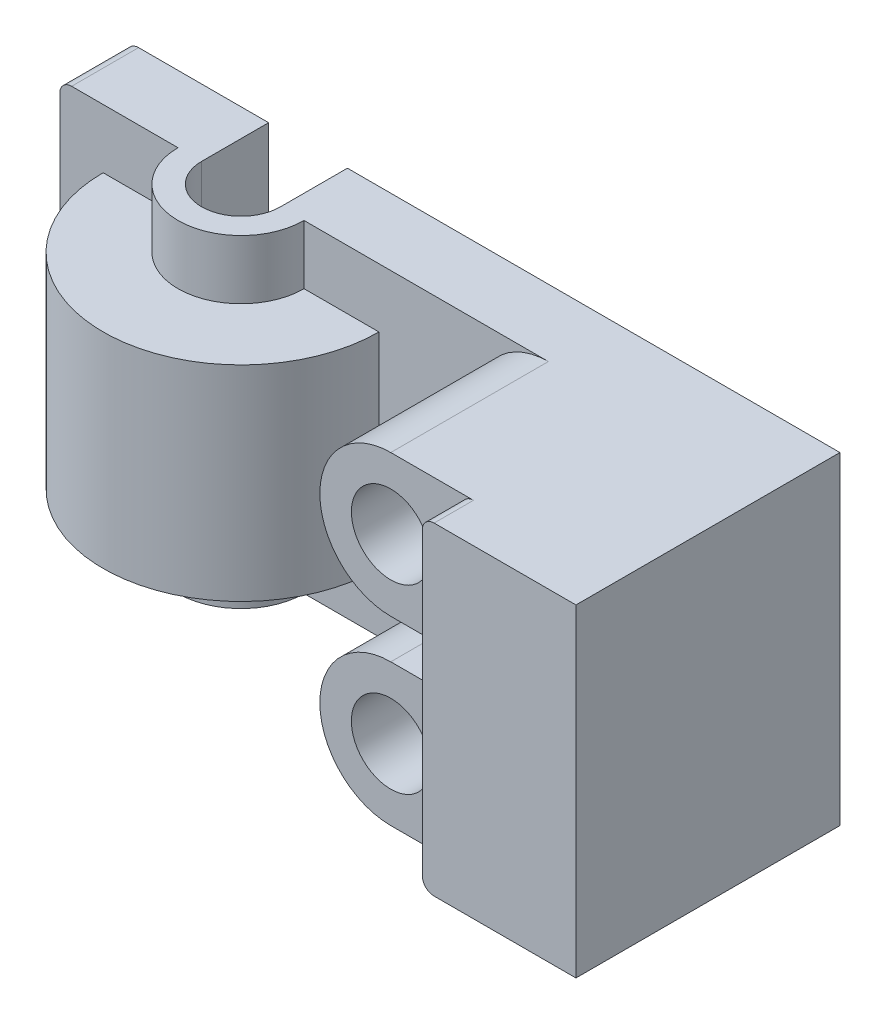
ISO-10303-21;
HEADER;
FILE_DESCRIPTION(('STEP AP214'),'2;1');
FILE_NAME('part.step','',(''),(''),'','','');
FILE_SCHEMA(('AUTOMOTIVE_DESIGN { 1 0 10303 214 1 1 1 1 }'));
ENDSEC;
DATA;
#1=APPLICATION_CONTEXT('core data for automotive mechanical design processes');
#2=APPLICATION_PROTOCOL_DEFINITION('international standard','automotive_design',2000,#1);
#3=PRODUCT_CONTEXT('',#1,'mechanical');
#4=PRODUCT('Part','Part','',(#3));
#5=PRODUCT_RELATED_PRODUCT_CATEGORY('part','',(#4));
#6=PRODUCT_DEFINITION_FORMATION('','',#4);
#7=PRODUCT_DEFINITION_CONTEXT('part definition',#1,'design');
#8=PRODUCT_DEFINITION('design','',#6,#7);
#9=PRODUCT_DEFINITION_SHAPE('','',#8);
#10=(LENGTH_UNIT() NAMED_UNIT(*) SI_UNIT(.MILLI.,.METRE.));
#11=(NAMED_UNIT(*) PLANE_ANGLE_UNIT() SI_UNIT($,.RADIAN.));
#12=(NAMED_UNIT(*) SI_UNIT($,.STERADIAN.) SOLID_ANGLE_UNIT());
#13=UNCERTAINTY_MEASURE_WITH_UNIT(LENGTH_MEASURE(1.E-05),#10,'distance_accuracy_value','');
#14=(GEOMETRIC_REPRESENTATION_CONTEXT(3) GLOBAL_UNCERTAINTY_ASSIGNED_CONTEXT((#13)) GLOBAL_UNIT_ASSIGNED_CONTEXT((#10,
#11,#12)) REPRESENTATION_CONTEXT('',''));
#15=CARTESIAN_POINT('',(0.,0.,0.));
#16=DIRECTION('',(0.,0.,1.));
#17=DIRECTION('',(1.,0.,0.));
#18=AXIS2_PLACEMENT_3D('',#15,#16,#17);
#19=CARTESIAN_POINT('',(0.,0.,17.));
#20=DIRECTION('',(0.,0.,1.));
#21=DIRECTION('',(1.,0.,0.));
#22=AXIS2_PLACEMENT_3D('',#19,#20,#21);
#23=PLANE('',#22);
#24=DIRECTION('',(1.,0.,0.));
#25=VECTOR('',#24,1.);
#26=CARTESIAN_POINT('',(118.,46.,17.));
#27=LINE('',#26,#25);
#28=CARTESIAN_POINT('',(118.,46.,17.));
#29=VERTEX_POINT('',#28);
#30=CARTESIAN_POINT('',(136.,46.,17.));
#31=VERTEX_POINT('',#30);
#32=EDGE_CURVE('E236',#29,#31,#27,.T.);
#33=ORIENTED_EDGE('',*,*,#32,.F.);
#34=CARTESIAN_POINT('',(118.,64.,17.));
#35=DIRECTION('',(0.,0.,1.));
#36=DIRECTION('',(1.,0.,0.));
#37=AXIS2_PLACEMENT_3D('',#34,#35,#36);
#38=CIRCLE('',#37,18.);
#39=CARTESIAN_POINT('',(118.,82.,17.));
#40=VERTEX_POINT('',#39);
#41=EDGE_CURVE('E566',#40,#29,#38,.T.);
#42=ORIENTED_EDGE('',*,*,#41,.F.);
#43=DIRECTION('',(-1.,0.,0.));
#44=VECTOR('',#43,1.);
#45=CARTESIAN_POINT('',(175.,82.,17.));
#46=LINE('',#45,#44);
#47=CARTESIAN_POINT('',(56.,82.,17.));
#48=VERTEX_POINT('',#47);
#49=EDGE_CURVE('E253',#40,#48,#46,.T.);
#50=ORIENTED_EDGE('',*,*,#49,.T.);
#51=DIRECTION('',(0.,-1.,0.));
#52=VECTOR('',#51,1.);
#53=CARTESIAN_POINT('',(56.,82.,17.));
#54=LINE('',#53,#52);
#55=CARTESIAN_POINT('',(56.,67.,17.));
#56=VERTEX_POINT('',#55);
#57=EDGE_CURVE('E391',#48,#56,#54,.T.);
#58=ORIENTED_EDGE('',*,*,#57,.T.);
#59=DIRECTION('',(-1.,0.,0.));
#60=VECTOR('',#59,1.);
#61=CARTESIAN_POINT('',(50.,67.,17.));
#62=LINE('',#61,#60);
#63=CARTESIAN_POINT('',(75.,67.,17.));
#64=VERTEX_POINT('',#63);
#65=EDGE_CURVE('E401',#64,#56,#62,.T.);
#66=ORIENTED_EDGE('',*,*,#65,.F.);
#67=DIRECTION('',(0.,-1.,0.));
#68=VECTOR('',#67,1.);
#69=CARTESIAN_POINT('',(75.,82.,17.));
#70=LINE('',#69,#68);
#71=CARTESIAN_POINT('',(75.,15.,17.));
#72=VERTEX_POINT('',#71);
#73=EDGE_CURVE('E285',#64,#72,#70,.T.);
#74=ORIENTED_EDGE('',*,*,#73,.T.);
#75=DIRECTION('',(1.,0.,0.));
#76=VECTOR('',#75,1.);
#77=CARTESIAN_POINT('',(50.,15.,17.));
#78=LINE('',#77,#76);
#79=CARTESIAN_POINT('',(56.,15.,17.));
#80=VERTEX_POINT('',#79);
#81=EDGE_CURVE('E415',#80,#72,#78,.T.);
#82=ORIENTED_EDGE('',*,*,#81,.F.);
#83=DIRECTION('',(0.,1.,0.));
#84=VECTOR('',#83,1.);
#85=CARTESIAN_POINT('',(56.,0.,17.));
#86=LINE('',#85,#84);
#87=CARTESIAN_POINT('',(56.,0.,17.));
#88=VERTEX_POINT('',#87);
#89=EDGE_CURVE('E383',#88,#80,#86,.T.);
#90=ORIENTED_EDGE('',*,*,#89,.F.);
#91=DIRECTION('',(1.,0.,0.));
#92=VECTOR('',#91,1.);
#93=CARTESIAN_POINT('',(0.,0.,17.));
#94=LINE('',#93,#92);
#95=CARTESIAN_POINT('',(118.,0.,17.));
#96=VERTEX_POINT('',#95);
#97=EDGE_CURVE('E251',#88,#96,#94,.T.);
#98=ORIENTED_EDGE('',*,*,#97,.T.);
#99=CARTESIAN_POINT('',(118.,18.,17.));
#100=DIRECTION('',(0.,0.,1.));
#101=DIRECTION('',(1.,0.,0.));
#102=AXIS2_PLACEMENT_3D('',#99,#100,#101);
#103=CIRCLE('',#102,18.);
#104=CARTESIAN_POINT('',(118.,36.,17.));
#105=VERTEX_POINT('',#104);
#106=EDGE_CURVE('E360',#105,#96,#103,.T.);
#107=ORIENTED_EDGE('',*,*,#106,.F.);
#108=DIRECTION('',(-1.,0.,0.));
#109=VECTOR('',#108,1.);
#110=CARTESIAN_POINT('',(118.,36.,17.));
#111=LINE('',#110,#109);
#112=CARTESIAN_POINT('',(136.,36.,17.));
#113=VERTEX_POINT('',#112);
#114=EDGE_CURVE('E366',#113,#105,#111,.T.);
#115=ORIENTED_EDGE('',*,*,#114,.F.);
#116=DIRECTION('',(0.,-1.,0.));
#117=VECTOR('',#116,1.);
#118=CARTESIAN_POINT('',(136.,79.,17.));
#119=LINE('',#118,#117);
#120=EDGE_CURVE('E322',#31,#113,#119,.T.);
#121=ORIENTED_EDGE('',*,*,#120,.F.);
#122=EDGE_LOOP('',(#33,#42,#50,#58,#66,#74,#82,#90,#98,#107,#115,#121));
#123=FACE_BOUND('',#122,.T.);
#124=ADVANCED_FACE('F50',(#123),#23,.T.);
#125=CARTESIAN_POINT('',(136.,79.,67.));
#126=DIRECTION('',(1.,0.,0.));
#127=DIRECTION('',(0.,0.,-1.));
#128=AXIS2_PLACEMENT_3D('',#125,#126,#127);
#129=PLANE('',#128);
#130=DIRECTION('',(0.,0.,-1.));
#131=VECTOR('',#130,1.);
#132=CARTESIAN_POINT('',(136.,46.,57.));
#133=LINE('',#132,#131);
#134=CARTESIAN_POINT('',(136.,46.,57.));
#135=VERTEX_POINT('',#134);
#136=EDGE_CURVE('E556',#135,#31,#133,.T.);
#137=ORIENTED_EDGE('',*,*,#136,.T.);
#138=ORIENTED_EDGE('',*,*,#120,.T.);
#139=DIRECTION('',(0.,0.,-1.));
#140=VECTOR('',#139,1.);
#141=CARTESIAN_POINT('',(136.,36.,57.));
#142=LINE('',#141,#140);
#143=CARTESIAN_POINT('',(136.,36.,57.));
#144=VERTEX_POINT('',#143);
#145=EDGE_CURVE('E351',#144,#113,#142,.T.);
#146=ORIENTED_EDGE('',*,*,#145,.F.);
#147=DIRECTION('',(0.,1.,0.));
#148=VECTOR('',#147,1.);
#149=CARTESIAN_POINT('',(136.,36.,57.));
#150=LINE('',#149,#148);
#151=CARTESIAN_POINT('',(136.,3.,57.));
#152=VERTEX_POINT('',#151);
#153=EDGE_CURVE('E353',#152,#144,#150,.T.);
#154=ORIENTED_EDGE('',*,*,#153,.F.);
#155=DIRECTION('',(0.,0.,-1.));
#156=VECTOR('',#155,1.);
#157=CARTESIAN_POINT('',(136.,3.,67.));
#158=LINE('',#157,#156);
#159=CARTESIAN_POINT('',(136.,3.,67.));
#160=VERTEX_POINT('',#159);
#161=EDGE_CURVE('E246',#160,#152,#158,.T.);
#162=ORIENTED_EDGE('',*,*,#161,.F.);
#163=DIRECTION('',(0.,-1.,0.));
#164=VECTOR('',#163,1.);
#165=CARTESIAN_POINT('',(136.,79.,67.));
#166=LINE('',#165,#164);
#167=CARTESIAN_POINT('',(136.,79.,67.));
#168=VERTEX_POINT('',#167);
#169=EDGE_CURVE('E328',#168,#160,#166,.T.);
#170=ORIENTED_EDGE('',*,*,#169,.F.);
#171=DIRECTION('',(0.,0.,-1.));
#172=VECTOR('',#171,1.);
#173=CARTESIAN_POINT('',(136.,79.,67.));
#174=LINE('',#173,#172);
#175=CARTESIAN_POINT('',(136.,79.,57.));
#176=VERTEX_POINT('',#175);
#177=EDGE_CURVE('E245',#168,#176,#174,.T.);
#178=ORIENTED_EDGE('',*,*,#177,.T.);
#179=DIRECTION('',(0.,1.,0.));
#180=VECTOR('',#179,1.);
#181=CARTESIAN_POINT('',(136.,46.,57.));
#182=LINE('',#181,#180);
#183=EDGE_CURVE('E65',#135,#176,#182,.T.);
#184=ORIENTED_EDGE('',*,*,#183,.F.);
#185=EDGE_LOOP('',(#137,#138,#146,#154,#162,#170,#178,#184));
#186=FACE_BOUND('',#185,.T.);
#187=ADVANCED_FACE('F349',(#186),#129,.F.);
#188=CARTESIAN_POINT('',(-3.,0.,17.));
#189=VERTEX_POINT('',#188);
#190=CARTESIAN_POINT('',(24.,0.,17.));
#191=VERTEX_POINT('',#190);
#192=EDGE_CURVE('E249',#189,#191,#94,.T.);
#193=ORIENTED_EDGE('',*,*,#192,.T.);
#194=DIRECTION('',(0.,1.,0.));
#195=VECTOR('',#194,1.);
#196=CARTESIAN_POINT('',(24.,0.,17.));
#197=LINE('',#196,#195);
#198=CARTESIAN_POINT('',(24.,15.,17.));
#199=VERTEX_POINT('',#198);
#200=EDGE_CURVE('E382',#191,#199,#197,.T.);
#201=ORIENTED_EDGE('',*,*,#200,.T.);
#202=DIRECTION('',(1.,0.,0.));
#203=VECTOR('',#202,1.);
#204=CARTESIAN_POINT('',(4.99999999999998,15.,16.9999999999998));
#205=LINE('',#204,#203);
#206=CARTESIAN_POINT('',(4.99999999999998,15.,16.9999999999998));
#207=VERTEX_POINT('',#206);
#208=EDGE_CURVE('E408',#207,#199,#205,.T.);
#209=ORIENTED_EDGE('',*,*,#208,.F.);
#210=DIRECTION('',(0.,-1.,0.));
#211=VECTOR('',#210,1.);
#212=CARTESIAN_POINT('',(4.99999999999997,82.,17.));
#213=LINE('',#212,#211);
#214=CARTESIAN_POINT('',(4.99999999999998,67.,17.));
#215=VERTEX_POINT('',#214);
#216=EDGE_CURVE('E293',#215,#207,#213,.T.);
#217=ORIENTED_EDGE('',*,*,#216,.F.);
#218=DIRECTION('',(-1.,0.,0.));
#219=VECTOR('',#218,1.);
#220=CARTESIAN_POINT('',(30.,67.,17.));
#221=LINE('',#220,#219);
#222=CARTESIAN_POINT('',(24.,67.,17.));
#223=VERTEX_POINT('',#222);
#224=EDGE_CURVE('E397',#223,#215,#221,.T.);
#225=ORIENTED_EDGE('',*,*,#224,.F.);
#226=DIRECTION('',(0.,-1.,0.));
#227=VECTOR('',#226,1.);
#228=CARTESIAN_POINT('',(24.,82.,17.));
#229=LINE('',#228,#227);
#230=CARTESIAN_POINT('',(24.,82.,17.));
#231=VERTEX_POINT('',#230);
#232=EDGE_CURVE('E400',#231,#223,#229,.T.);
#233=ORIENTED_EDGE('',*,*,#232,.F.);
#234=CARTESIAN_POINT('',(-3.,82.,17.));
#235=VERTEX_POINT('',#234);
#236=EDGE_CURVE('E254',#231,#235,#46,.T.);
#237=ORIENTED_EDGE('',*,*,#236,.T.);
#238=CARTESIAN_POINT('',(-3.,79.,17.));
#239=DIRECTION('',(0.,0.,1.));
#240=DIRECTION('',(1.,0.,0.));
#241=AXIS2_PLACEMENT_3D('',#238,#239,#240);
#242=CIRCLE('',#241,3.);
#243=CARTESIAN_POINT('',(-6.,79.,17.));
#244=VERTEX_POINT('',#243);
#245=EDGE_CURVE('E291',#235,#244,#242,.T.);
#246=ORIENTED_EDGE('',*,*,#245,.T.);
#247=DIRECTION('',(0.,-1.,0.));
#248=VECTOR('',#247,1.);
#249=CARTESIAN_POINT('',(-6.,79.,17.));
#250=LINE('',#249,#248);
#251=CARTESIAN_POINT('',(-6.,3.,17.));
#252=VERTEX_POINT('',#251);
#253=EDGE_CURVE('E307',#244,#252,#250,.T.);
#254=ORIENTED_EDGE('',*,*,#253,.T.);
#255=CARTESIAN_POINT('',(-3.,3.,17.));
#256=DIRECTION('',(0.,0.,1.));
#257=DIRECTION('',(1.,0.,0.));
#258=AXIS2_PLACEMENT_3D('',#255,#256,#257);
#259=CIRCLE('',#258,3.);
#260=EDGE_CURVE('E297',#252,#189,#259,.T.);
#261=ORIENTED_EDGE('',*,*,#260,.T.);
#262=EDGE_LOOP('',(#193,#201,#209,#217,#225,#233,#237,#246,#254,#261));
#263=FACE_BOUND('',#262,.T.);
#264=ADVANCED_FACE('F444',(#263),#23,.T.);
#265=CARTESIAN_POINT('',(40.,15.,17.));
#266=DIRECTION('',(0.,-1.,0.));
#267=DIRECTION('',(0.,0.,-1.));
#268=AXIS2_PLACEMENT_3D('',#265,#266,#267);
#269=PLANE('',#268);
#270=ORIENTED_EDGE('',*,*,#208,.T.);
#271=CARTESIAN_POINT('',(40.,15.,17.));
#272=DIRECTION('',(0.,-1.,0.));
#273=DIRECTION('',(0.,0.,-1.));
#274=AXIS2_PLACEMENT_3D('',#271,#272,#273);
#275=CIRCLE('',#274,16.);
#276=EDGE_CURVE('E374',#80,#199,#275,.T.);
#277=ORIENTED_EDGE('',*,*,#276,.F.);
#278=ORIENTED_EDGE('',*,*,#81,.T.);
#279=CARTESIAN_POINT('',(40.,15.,17.));
#280=DIRECTION('',(0.,-1.,0.));
#281=DIRECTION('',(0.,0.,-1.));
#282=AXIS2_PLACEMENT_3D('',#279,#280,#281);
#283=CIRCLE('',#282,35.);
#284=EDGE_CURVE('E406',#72,#207,#283,.T.);
#285=ORIENTED_EDGE('',*,*,#284,.T.);
#286=EDGE_LOOP('',(#270,#277,#278,#285));
#287=FACE_BOUND('',#286,.T.);
#288=ADVANCED_FACE('F462',(#287),#269,.T.);
#289=CARTESIAN_POINT('',(40.,67.,17.));
#290=DIRECTION('',(0.,1.,0.));
#291=DIRECTION('',(0.,0.,1.));
#292=AXIS2_PLACEMENT_3D('',#289,#290,#291);
#293=PLANE('',#292);
#294=ORIENTED_EDGE('',*,*,#65,.T.);
#295=CARTESIAN_POINT('',(40.,67.,17.));
#296=DIRECTION('',(0.,1.,0.));
#297=DIRECTION('',(0.,0.,1.));
#298=AXIS2_PLACEMENT_3D('',#295,#296,#297);
#299=CIRCLE('',#298,16.);
#300=EDGE_CURVE('E390',#223,#56,#299,.T.);
#301=ORIENTED_EDGE('',*,*,#300,.F.);
#302=ORIENTED_EDGE('',*,*,#224,.T.);
#303=CARTESIAN_POINT('',(40.,67.,17.));
#304=DIRECTION('',(0.,1.,0.));
#305=DIRECTION('',(0.,0.,1.));
#306=AXIS2_PLACEMENT_3D('',#303,#304,#305);
#307=CIRCLE('',#306,35.);
#308=EDGE_CURVE('E402',#215,#64,#307,.T.);
#309=ORIENTED_EDGE('',*,*,#308,.T.);
#310=EDGE_LOOP('',(#294,#301,#302,#309));
#311=FACE_BOUND('',#310,.T.);
#312=ADVANCED_FACE('F455',(#311),#293,.T.);
#313=CARTESIAN_POINT('',(40.,82.,17.));
#314=DIRECTION('',(0.,-1.,0.));
#315=DIRECTION('',(0.,0.,-1.));
#316=AXIS2_PLACEMENT_3D('',#313,#314,#315);
#317=CYLINDRICAL_SURFACE('',#316,35.);
#318=ORIENTED_EDGE('',*,*,#73,.F.);
#319=ORIENTED_EDGE('',*,*,#308,.F.);
#320=ORIENTED_EDGE('',*,*,#216,.T.);
#321=ORIENTED_EDGE('',*,*,#284,.F.);
#322=EDGE_LOOP('',(#318,#319,#320,#321));
#323=FACE_BOUND('',#322,.T.);
#324=ADVANCED_FACE('F463',(#323),#317,.T.);
#325=CARTESIAN_POINT('',(40.,82.,17.));
#326=DIRECTION('',(0.,-1.,0.));
#327=DIRECTION('',(0.,0.,-1.));
#328=AXIS2_PLACEMENT_3D('',#325,#326,#327);
#329=CYLINDRICAL_SURFACE('',#328,10.);
#330=DIRECTION('',(0.,-1.,0.));
#331=VECTOR('',#330,1.);
#332=CARTESIAN_POINT('',(50.,82.,17.));
#333=LINE('',#332,#331);
#334=CARTESIAN_POINT('',(50.,82.,17.));
#335=VERTEX_POINT('',#334);
#336=CARTESIAN_POINT('',(50.,0.,17.));
#337=VERTEX_POINT('',#336);
#338=EDGE_CURVE('E278',#335,#337,#333,.T.);
#339=ORIENTED_EDGE('',*,*,#338,.T.);
#340=CARTESIAN_POINT('',(40.,0.,17.));
#341=DIRECTION('',(0.,1.,0.));
#342=DIRECTION('',(0.,0.,-1.));
#343=AXIS2_PLACEMENT_3D('',#340,#341,#342);
#344=CIRCLE('',#343,10.);
#345=CARTESIAN_POINT('',(30.,0.,17.));
#346=VERTEX_POINT('',#345);
#347=EDGE_CURVE('E376',#346,#337,#344,.T.);
#348=ORIENTED_EDGE('',*,*,#347,.F.);
#349=DIRECTION('',(0.,-1.,0.));
#350=VECTOR('',#349,1.);
#351=CARTESIAN_POINT('',(30.,82.,17.));
#352=LINE('',#351,#350);
#353=CARTESIAN_POINT('',(30.,82.,17.));
#354=VERTEX_POINT('',#353);
#355=EDGE_CURVE('E282',#354,#346,#352,.T.);
#356=ORIENTED_EDGE('',*,*,#355,.F.);
#357=CARTESIAN_POINT('',(40.,82.,17.));
#358=DIRECTION('',(0.,-1.,0.));
#359=DIRECTION('',(0.,0.,1.));
#360=AXIS2_PLACEMENT_3D('',#357,#358,#359);
#361=CIRCLE('',#360,10.);
#362=EDGE_CURVE('E387',#335,#354,#361,.T.);
#363=ORIENTED_EDGE('',*,*,#362,.F.);
#364=EDGE_LOOP('',(#339,#348,#356,#363));
#365=FACE_BOUND('',#364,.T.);
#366=ADVANCED_FACE('F430',(#365),#329,.F.);
#367=CARTESIAN_POINT('',(0.,0.,0.));
#368=DIRECTION('',(0.,0.,1.));
#369=DIRECTION('',(1.,0.,0.));
#370=AXIS2_PLACEMENT_3D('',#367,#368,#369);
#371=PLANE('',#370);
#372=DIRECTION('',(1.,0.,0.));
#373=VECTOR('',#372,1.);
#374=CARTESIAN_POINT('',(0.,0.,0.));
#375=LINE('',#374,#373);
#376=CARTESIAN_POINT('',(50.,0.,0.));
#377=VERTEX_POINT('',#376);
#378=CARTESIAN_POINT('',(175.,0.,0.));
#379=VERTEX_POINT('',#378);
#380=EDGE_CURVE('E241',#377,#379,#375,.T.);
#381=ORIENTED_EDGE('',*,*,#380,.F.);
#382=DIRECTION('',(0.,-1.,0.));
#383=VECTOR('',#382,1.);
#384=CARTESIAN_POINT('',(50.,82.,0.));
#385=LINE('',#384,#383);
#386=CARTESIAN_POINT('',(50.,82.,0.));
#387=VERTEX_POINT('',#386);
#388=EDGE_CURVE('E273',#387,#377,#385,.T.);
#389=ORIENTED_EDGE('',*,*,#388,.F.);
#390=DIRECTION('',(-1.,0.,0.));
#391=VECTOR('',#390,1.);
#392=CARTESIAN_POINT('',(175.,82.,0.));
#393=LINE('',#392,#391);
#394=CARTESIAN_POINT('',(175.,82.,0.));
#395=VERTEX_POINT('',#394);
#396=EDGE_CURVE('E263',#395,#387,#393,.T.);
#397=ORIENTED_EDGE('',*,*,#396,.F.);
#398=DIRECTION('',(0.,1.,0.));
#399=VECTOR('',#398,1.);
#400=CARTESIAN_POINT('',(175.,0.,0.));
#401=LINE('',#400,#399);
#402=EDGE_CURVE('E257',#379,#395,#401,.T.);
#403=ORIENTED_EDGE('',*,*,#402,.F.);
#404=EDGE_LOOP('',(#381,#389,#397,#403));
#405=FACE_BOUND('',#404,.T.);
#406=ADVANCED_FACE('F274',(#405),#371,.F.);
#407=CARTESIAN_POINT('',(0.,0.,17.));
#408=DIRECTION('',(0.,1.,0.));
#409=DIRECTION('',(0.,0.,1.));
#410=AXIS2_PLACEMENT_3D('',#407,#408,#409);
#411=PLANE('',#410);
#412=DIRECTION('',(0.,0.,-1.));
#413=VECTOR('',#412,1.);
#414=CARTESIAN_POINT('',(30.,0.,17.));
#415=LINE('',#414,#413);
#416=CARTESIAN_POINT('',(30.,0.,0.));
#417=VERTEX_POINT('',#416);
#418=EDGE_CURVE('E414',#346,#417,#415,.T.);
#419=ORIENTED_EDGE('',*,*,#418,.F.);
#420=ORIENTED_EDGE('',*,*,#347,.T.);
#421=DIRECTION('',(0.,0.,1.));
#422=VECTOR('',#421,1.);
#423=CARTESIAN_POINT('',(50.,0.,17.));
#424=LINE('',#423,#422);
#425=EDGE_CURVE('E416',#377,#337,#424,.T.);
#426=ORIENTED_EDGE('',*,*,#425,.F.);
#427=ORIENTED_EDGE('',*,*,#380,.T.);
#428=DIRECTION('',(0.,0.,-1.));
#429=VECTOR('',#428,1.);
#430=CARTESIAN_POINT('',(175.,0.,17.));
#431=LINE('',#430,#429);
#432=CARTESIAN_POINT('',(175.,0.,67.));
#433=VERTEX_POINT('',#432);
#434=EDGE_CURVE('E11',#433,#379,#431,.T.);
#435=ORIENTED_EDGE('',*,*,#434,.F.);
#436=DIRECTION('',(1.,0.,0.));
#437=VECTOR('',#436,1.);
#438=CARTESIAN_POINT('',(175.,0.,67.));
#439=LINE('',#438,#437);
#440=CARTESIAN_POINT('',(139.,0.,67.));
#441=VERTEX_POINT('',#440);
#442=EDGE_CURVE('E327',#441,#433,#439,.T.);
#443=ORIENTED_EDGE('',*,*,#442,.F.);
#444=DIRECTION('',(0.,0.,-1.));
#445=VECTOR('',#444,1.);
#446=CARTESIAN_POINT('',(139.,0.,67.));
#447=LINE('',#446,#445);
#448=CARTESIAN_POINT('',(139.,0.,57.));
#449=VERTEX_POINT('',#448);
#450=EDGE_CURVE('E334',#441,#449,#447,.T.);
#451=ORIENTED_EDGE('',*,*,#450,.T.);
#452=DIRECTION('',(1.,0.,0.));
#453=VECTOR('',#452,1.);
#454=CARTESIAN_POINT('',(118.,0.,57.));
#455=LINE('',#454,#453);
#456=CARTESIAN_POINT('',(118.,0.,57.));
#457=VERTEX_POINT('',#456);
#458=EDGE_CURVE('E67',#457,#449,#455,.T.);
#459=ORIENTED_EDGE('',*,*,#458,.F.);
#460=DIRECTION('',(0.,0.,-1.));
#461=VECTOR('',#460,1.);
#462=CARTESIAN_POINT('',(118.,0.,57.));
#463=LINE('',#462,#461);
#464=EDGE_CURVE('E362',#457,#96,#463,.T.);
#465=ORIENTED_EDGE('',*,*,#464,.T.);
#466=ORIENTED_EDGE('',*,*,#97,.F.);
#467=CARTESIAN_POINT('',(40.,0.,17.));
#468=DIRECTION('',(0.,-1.,0.));
#469=DIRECTION('',(0.,0.,-1.));
#470=AXIS2_PLACEMENT_3D('',#467,#468,#469);
#471=CIRCLE('',#470,16.);
#472=EDGE_CURVE('E378',#88,#191,#471,.T.);
#473=ORIENTED_EDGE('',*,*,#472,.T.);
#474=ORIENTED_EDGE('',*,*,#192,.F.);
#475=DIRECTION('',(0.,0.,1.));
#476=VECTOR('',#475,1.);
#477=CARTESIAN_POINT('',(-3.,0.,17.));
#478=LINE('',#477,#476);
#479=CARTESIAN_POINT('',(-3.,0.,0.));
#480=VERTEX_POINT('',#479);
#481=EDGE_CURVE('E317',#480,#189,#478,.T.);
#482=ORIENTED_EDGE('',*,*,#481,.F.);
#483=EDGE_CURVE('E242',#480,#417,#375,.T.);
#484=ORIENTED_EDGE('',*,*,#483,.T.);
#485=EDGE_LOOP('',(#419,#420,#426,#427,#435,#443,#451,#459,#465,#466,#473,#474,#482,#484));
#486=FACE_BOUND('',#485,.T.);
#487=ADVANCED_FACE('F47',(#486),#411,.F.);
#488=CARTESIAN_POINT('',(175.,0.,17.));
#489=DIRECTION('',(-1.,0.,0.));
#490=DIRECTION('',(0.,0.,1.));
#491=AXIS2_PLACEMENT_3D('',#488,#489,#490);
#492=PLANE('',#491);
#493=ORIENTED_EDGE('',*,*,#402,.T.);
#494=DIRECTION('',(0.,0.,-1.));
#495=VECTOR('',#494,1.);
#496=CARTESIAN_POINT('',(175.,82.,17.));
#497=LINE('',#496,#495);
#498=CARTESIAN_POINT('',(175.,82.,67.));
#499=VERTEX_POINT('',#498);
#500=EDGE_CURVE('E54',#499,#395,#497,.T.);
#501=ORIENTED_EDGE('',*,*,#500,.F.);
#502=DIRECTION('',(0.,1.,0.));
#503=VECTOR('',#502,1.);
#504=CARTESIAN_POINT('',(175.,82.,67.));
#505=LINE('',#504,#503);
#506=EDGE_CURVE('E331',#433,#499,#505,.T.);
#507=ORIENTED_EDGE('',*,*,#506,.F.);
#508=ORIENTED_EDGE('',*,*,#434,.T.);
#509=EDGE_LOOP('',(#493,#501,#507,#508));
#510=FACE_BOUND('',#509,.T.);
#511=ADVANCED_FACE('F542',(#510),#492,.F.);
#512=CARTESIAN_POINT('',(175.,82.,17.));
#513=DIRECTION('',(0.,-1.,0.));
#514=DIRECTION('',(0.,0.,-1.));
#515=AXIS2_PLACEMENT_3D('',#512,#513,#514);
#516=PLANE('',#515);
#517=ORIENTED_EDGE('',*,*,#49,.F.);
#518=DIRECTION('',(0.,0.,-1.));
#519=VECTOR('',#518,1.);
#520=CARTESIAN_POINT('',(118.,82.,57.));
#521=LINE('',#520,#519);
#522=CARTESIAN_POINT('',(118.,82.,57.));
#523=VERTEX_POINT('',#522);
#524=EDGE_CURVE('E227',#523,#40,#521,.T.);
#525=ORIENTED_EDGE('',*,*,#524,.F.);
#526=DIRECTION('',(-1.,0.,0.));
#527=VECTOR('',#526,1.);
#528=CARTESIAN_POINT('',(118.,82.,57.));
#529=LINE('',#528,#527);
#530=CARTESIAN_POINT('',(139.,82.,57.));
#531=VERTEX_POINT('',#530);
#532=EDGE_CURVE('E223',#531,#523,#529,.T.);
#533=ORIENTED_EDGE('',*,*,#532,.F.);
#534=DIRECTION('',(0.,0.,-1.));
#535=VECTOR('',#534,1.);
#536=CARTESIAN_POINT('',(139.,82.,67.));
#537=LINE('',#536,#535);
#538=CARTESIAN_POINT('',(139.,82.,67.));
#539=VERTEX_POINT('',#538);
#540=EDGE_CURVE('E228',#539,#531,#537,.T.);
#541=ORIENTED_EDGE('',*,*,#540,.F.);
#542=DIRECTION('',(-1.,0.,0.));
#543=VECTOR('',#542,1.);
#544=CARTESIAN_POINT('',(175.,82.,67.));
#545=LINE('',#544,#543);
#546=EDGE_CURVE('E268',#499,#539,#545,.T.);
#547=ORIENTED_EDGE('',*,*,#546,.F.);
#548=ORIENTED_EDGE('',*,*,#500,.T.);
#549=ORIENTED_EDGE('',*,*,#396,.T.);
#550=DIRECTION('',(0.,0.,1.));
#551=VECTOR('',#550,1.);
#552=CARTESIAN_POINT('',(50.,82.,17.));
#553=LINE('',#552,#551);
#554=EDGE_CURVE('E289',#387,#335,#553,.T.);
#555=ORIENTED_EDGE('',*,*,#554,.T.);
#556=ORIENTED_EDGE('',*,*,#362,.T.);
#557=DIRECTION('',(0.,0.,-1.));
#558=VECTOR('',#557,1.);
#559=CARTESIAN_POINT('',(30.,82.,17.));
#560=LINE('',#559,#558);
#561=CARTESIAN_POINT('',(30.,82.,0.));
#562=VERTEX_POINT('',#561);
#563=EDGE_CURVE('E412',#354,#562,#560,.T.);
#564=ORIENTED_EDGE('',*,*,#563,.T.);
#565=CARTESIAN_POINT('',(-3.,82.,0.));
#566=VERTEX_POINT('',#565);
#567=EDGE_CURVE('E259',#562,#566,#393,.T.);
#568=ORIENTED_EDGE('',*,*,#567,.T.);
#569=DIRECTION('',(0.,0.,-1.));
#570=VECTOR('',#569,1.);
#571=CARTESIAN_POINT('',(-3.,82.,0.));
#572=LINE('',#571,#570);
#573=EDGE_CURVE('E318',#235,#566,#572,.T.);
#574=ORIENTED_EDGE('',*,*,#573,.F.);
#575=ORIENTED_EDGE('',*,*,#236,.F.);
#576=CARTESIAN_POINT('',(40.,82.,17.));
#577=DIRECTION('',(0.,1.,0.));
#578=DIRECTION('',(0.,0.,1.));
#579=AXIS2_PLACEMENT_3D('',#576,#577,#578);
#580=CIRCLE('',#579,16.);
#581=EDGE_CURVE('E389',#231,#48,#580,.T.);
#582=ORIENTED_EDGE('',*,*,#581,.T.);
#583=EDGE_LOOP('',(#517,#525,#533,#541,#547,#548,#549,#555,#556,#564,#568,#574,#575,#582));
#584=FACE_BOUND('',#583,.T.);
#585=ADVANCED_FACE('F221',(#584),#516,.F.);
#586=ORIENTED_EDGE('',*,*,#567,.F.);
#587=DIRECTION('',(0.,-1.,0.));
#588=VECTOR('',#587,1.);
#589=CARTESIAN_POINT('',(30.,82.,0.));
#590=LINE('',#589,#588);
#591=EDGE_CURVE('E279',#562,#417,#590,.T.);
#592=ORIENTED_EDGE('',*,*,#591,.T.);
#593=ORIENTED_EDGE('',*,*,#483,.F.);
#594=CARTESIAN_POINT('',(-3.,3.,0.));
#595=DIRECTION('',(0.,0.,1.));
#596=DIRECTION('',(1.,0.,0.));
#597=AXIS2_PLACEMENT_3D('',#594,#595,#596);
#598=CIRCLE('',#597,3.);
#599=CARTESIAN_POINT('',(-6.,3.,0.));
#600=VERTEX_POINT('',#599);
#601=EDGE_CURVE('E303',#600,#480,#598,.T.);
#602=ORIENTED_EDGE('',*,*,#601,.F.);
#603=DIRECTION('',(0.,-1.,0.));
#604=VECTOR('',#603,1.);
#605=CARTESIAN_POINT('',(-6.,79.,0.));
#606=LINE('',#605,#604);
#607=CARTESIAN_POINT('',(-6.,79.,0.));
#608=VERTEX_POINT('',#607);
#609=EDGE_CURVE('E299',#608,#600,#606,.T.);
#610=ORIENTED_EDGE('',*,*,#609,.F.);
#611=CARTESIAN_POINT('',(-3.,79.,0.));
#612=DIRECTION('',(0.,0.,1.));
#613=DIRECTION('',(1.,0.,0.));
#614=AXIS2_PLACEMENT_3D('',#611,#612,#613);
#615=CIRCLE('',#614,3.);
#616=EDGE_CURVE('E298',#566,#608,#615,.T.);
#617=ORIENTED_EDGE('',*,*,#616,.F.);
#618=EDGE_LOOP('',(#586,#592,#593,#602,#610,#617));
#619=FACE_BOUND('',#618,.T.);
#620=ADVANCED_FACE('F432',(#619),#371,.F.);
#621=CARTESIAN_POINT('',(139.,79.,67.));
#622=DIRECTION('',(0.,0.,-1.));
#623=DIRECTION('',(-1.,0.,0.));
#624=AXIS2_PLACEMENT_3D('',#621,#622,#623);
#625=CYLINDRICAL_SURFACE('',#624,3.);
#626=ORIENTED_EDGE('',*,*,#540,.T.);
#627=CARTESIAN_POINT('',(139.,79.,57.));
#628=DIRECTION('',(0.,0.,-1.));
#629=DIRECTION('',(1.,0.,0.));
#630=AXIS2_PLACEMENT_3D('',#627,#628,#629);
#631=CIRCLE('',#630,3.);
#632=EDGE_CURVE('E229',#176,#531,#631,.T.);
#633=ORIENTED_EDGE('',*,*,#632,.F.);
#634=ORIENTED_EDGE('',*,*,#177,.F.);
#635=CARTESIAN_POINT('',(139.,79.,67.));
#636=DIRECTION('',(0.,0.,1.));
#637=DIRECTION('',(1.,0.,0.));
#638=AXIS2_PLACEMENT_3D('',#635,#636,#637);
#639=CIRCLE('',#638,3.);
#640=EDGE_CURVE('E237',#539,#168,#639,.T.);
#641=ORIENTED_EDGE('',*,*,#640,.F.);
#642=EDGE_LOOP('',(#626,#633,#634,#641));
#643=FACE_BOUND('',#642,.T.);
#644=ADVANCED_FACE('F238',(#643),#625,.T.);
#645=CARTESIAN_POINT('',(139.,3.,67.));
#646=DIRECTION('',(0.,0.,-1.));
#647=DIRECTION('',(-1.,0.,0.));
#648=AXIS2_PLACEMENT_3D('',#645,#646,#647);
#649=CYLINDRICAL_SURFACE('',#648,3.);
#650=ORIENTED_EDGE('',*,*,#161,.T.);
#651=CARTESIAN_POINT('',(139.,3.,57.));
#652=DIRECTION('',(0.,0.,-1.));
#653=DIRECTION('',(1.,0.,0.));
#654=AXIS2_PLACEMENT_3D('',#651,#652,#653);
#655=CIRCLE('',#654,3.);
#656=EDGE_CURVE('E343',#449,#152,#655,.T.);
#657=ORIENTED_EDGE('',*,*,#656,.F.);
#658=ORIENTED_EDGE('',*,*,#450,.F.);
#659=CARTESIAN_POINT('',(139.,3.,67.));
#660=DIRECTION('',(0.,0.,1.));
#661=DIRECTION('',(1.,0.,0.));
#662=AXIS2_PLACEMENT_3D('',#659,#660,#661);
#663=CIRCLE('',#662,3.);
#664=EDGE_CURVE('E326',#160,#441,#663,.T.);
#665=ORIENTED_EDGE('',*,*,#664,.F.);
#666=EDGE_LOOP('',(#650,#657,#658,#665));
#667=FACE_BOUND('',#666,.T.);
#668=ADVANCED_FACE('F345',(#667),#649,.T.);
#669=CARTESIAN_POINT('',(139.,79.,67.));
#670=DIRECTION('',(0.,0.,1.));
#671=DIRECTION('',(1.,0.,0.));
#672=AXIS2_PLACEMENT_3D('',#669,#670,#671);
#673=PLANE('',#672);
#674=ORIENTED_EDGE('',*,*,#546,.T.);
#675=ORIENTED_EDGE('',*,*,#640,.T.);
#676=ORIENTED_EDGE('',*,*,#169,.T.);
#677=ORIENTED_EDGE('',*,*,#664,.T.);
#678=ORIENTED_EDGE('',*,*,#442,.T.);
#679=ORIENTED_EDGE('',*,*,#506,.T.);
#680=EDGE_LOOP('',(#674,#675,#676,#677,#678,#679));
#681=FACE_BOUND('',#680,.T.);
#682=ADVANCED_FACE('F531',(#681),#673,.T.);
#683=CARTESIAN_POINT('',(-3.,79.,0.));
#684=DIRECTION('',(0.,0.,1.));
#685=DIRECTION('',(1.,0.,0.));
#686=AXIS2_PLACEMENT_3D('',#683,#684,#685);
#687=CYLINDRICAL_SURFACE('',#686,3.);
#688=ORIENTED_EDGE('',*,*,#245,.F.);
#689=ORIENTED_EDGE('',*,*,#573,.T.);
#690=ORIENTED_EDGE('',*,*,#616,.T.);
#691=DIRECTION('',(0.,0.,1.));
#692=VECTOR('',#691,1.);
#693=CARTESIAN_POINT('',(-6.,79.,0.));
#694=LINE('',#693,#692);
#695=EDGE_CURVE('E306',#608,#244,#694,.T.);
#696=ORIENTED_EDGE('',*,*,#695,.T.);
#697=EDGE_LOOP('',(#688,#689,#690,#696));
#698=FACE_BOUND('',#697,.T.);
#699=ADVANCED_FACE('F437',(#698),#687,.T.);
#700=CARTESIAN_POINT('',(-3.,3.,0.));
#701=DIRECTION('',(0.,0.,1.));
#702=DIRECTION('',(1.,0.,0.));
#703=AXIS2_PLACEMENT_3D('',#700,#701,#702);
#704=CYLINDRICAL_SURFACE('',#703,3.);
#705=ORIENTED_EDGE('',*,*,#260,.F.);
#706=DIRECTION('',(0.,0.,1.));
#707=VECTOR('',#706,1.);
#708=CARTESIAN_POINT('',(-6.,3.,0.));
#709=LINE('',#708,#707);
#710=EDGE_CURVE('E313',#600,#252,#709,.T.);
#711=ORIENTED_EDGE('',*,*,#710,.F.);
#712=ORIENTED_EDGE('',*,*,#601,.T.);
#713=ORIENTED_EDGE('',*,*,#481,.T.);
#714=EDGE_LOOP('',(#705,#711,#712,#713));
#715=FACE_BOUND('',#714,.T.);
#716=ADVANCED_FACE('F524',(#715),#704,.T.);
#717=CARTESIAN_POINT('',(-6.,79.,0.));
#718=DIRECTION('',(-1.,0.,0.));
#719=DIRECTION('',(0.,-1.,0.));
#720=AXIS2_PLACEMENT_3D('',#717,#718,#719);
#721=PLANE('',#720);
#722=ORIENTED_EDGE('',*,*,#253,.F.);
#723=ORIENTED_EDGE('',*,*,#695,.F.);
#724=ORIENTED_EDGE('',*,*,#609,.T.);
#725=ORIENTED_EDGE('',*,*,#710,.T.);
#726=EDGE_LOOP('',(#722,#723,#724,#725));
#727=FACE_BOUND('',#726,.T.);
#728=ADVANCED_FACE('F517',(#727),#721,.T.);
#729=CARTESIAN_POINT('',(50.,82.,17.));
#730=DIRECTION('',(1.,0.,0.));
#731=DIRECTION('',(0.,0.,-1.));
#732=AXIS2_PLACEMENT_3D('',#729,#730,#731);
#733=PLANE('',#732);
#734=ORIENTED_EDGE('',*,*,#425,.T.);
#735=ORIENTED_EDGE('',*,*,#338,.F.);
#736=ORIENTED_EDGE('',*,*,#554,.F.);
#737=ORIENTED_EDGE('',*,*,#388,.T.);
#738=EDGE_LOOP('',(#734,#735,#736,#737));
#739=FACE_BOUND('',#738,.T.);
#740=ADVANCED_FACE('F423',(#739),#733,.F.);
#741=CARTESIAN_POINT('',(30.,82.,17.));
#742=DIRECTION('',(-1.,0.,0.));
#743=DIRECTION('',(0.,0.,1.));
#744=AXIS2_PLACEMENT_3D('',#741,#742,#743);
#745=PLANE('',#744);
#746=ORIENTED_EDGE('',*,*,#418,.T.);
#747=ORIENTED_EDGE('',*,*,#591,.F.);
#748=ORIENTED_EDGE('',*,*,#563,.F.);
#749=ORIENTED_EDGE('',*,*,#355,.T.);
#750=EDGE_LOOP('',(#746,#747,#748,#749));
#751=FACE_BOUND('',#750,.T.);
#752=ADVANCED_FACE('F520',(#751),#745,.F.);
#753=CARTESIAN_POINT('',(40.,82.,17.));
#754=DIRECTION('',(0.,-1.,0.));
#755=DIRECTION('',(0.,0.,-1.));
#756=AXIS2_PLACEMENT_3D('',#753,#754,#755);
#757=CYLINDRICAL_SURFACE('',#756,16.);
#758=ORIENTED_EDGE('',*,*,#300,.T.);
#759=ORIENTED_EDGE('',*,*,#57,.F.);
#760=ORIENTED_EDGE('',*,*,#581,.F.);
#761=ORIENTED_EDGE('',*,*,#232,.T.);
#762=EDGE_LOOP('',(#758,#759,#760,#761));
#763=FACE_BOUND('',#762,.T.);
#764=ADVANCED_FACE('F448',(#763),#757,.T.);
#765=CARTESIAN_POINT('',(40.,0.,17.));
#766=DIRECTION('',(0.,1.,0.));
#767=DIRECTION('',(0.,0.,1.));
#768=AXIS2_PLACEMENT_3D('',#765,#766,#767);
#769=CYLINDRICAL_SURFACE('',#768,16.);
#770=ORIENTED_EDGE('',*,*,#276,.T.);
#771=ORIENTED_EDGE('',*,*,#200,.F.);
#772=ORIENTED_EDGE('',*,*,#472,.F.);
#773=ORIENTED_EDGE('',*,*,#89,.T.);
#774=EDGE_LOOP('',(#770,#771,#772,#773));
#775=FACE_BOUND('',#774,.T.);
#776=ADVANCED_FACE('F695',(#775),#769,.T.);
#777=CARTESIAN_POINT('',(118.,36.,57.));
#778=DIRECTION('',(0.,-1.,0.));
#779=DIRECTION('',(0.,0.,-1.));
#780=AXIS2_PLACEMENT_3D('',#777,#778,#779);
#781=PLANE('',#780);
#782=ORIENTED_EDGE('',*,*,#114,.T.);
#783=DIRECTION('',(0.,0.,-1.));
#784=VECTOR('',#783,1.);
#785=CARTESIAN_POINT('',(118.,36.,57.));
#786=LINE('',#785,#784);
#787=CARTESIAN_POINT('',(118.,36.,57.));
#788=VERTEX_POINT('',#787);
#789=EDGE_CURVE('E371',#788,#105,#786,.T.);
#790=ORIENTED_EDGE('',*,*,#789,.F.);
#791=DIRECTION('',(-1.,0.,0.));
#792=VECTOR('',#791,1.);
#793=CARTESIAN_POINT('',(118.,36.,57.));
#794=LINE('',#793,#792);
#795=EDGE_CURVE('E354',#144,#788,#794,.T.);
#796=ORIENTED_EDGE('',*,*,#795,.F.);
#797=ORIENTED_EDGE('',*,*,#145,.T.);
#798=EDGE_LOOP('',(#782,#790,#796,#797));
#799=FACE_BOUND('',#798,.T.);
#800=ADVANCED_FACE('F477',(#799),#781,.F.);
#801=CARTESIAN_POINT('',(118.,18.,57.));
#802=DIRECTION('',(0.,0.,-1.));
#803=DIRECTION('',(-1.,0.,0.));
#804=AXIS2_PLACEMENT_3D('',#801,#802,#803);
#805=CYLINDRICAL_SURFACE('',#804,18.);
#806=ORIENTED_EDGE('',*,*,#106,.T.);
#807=ORIENTED_EDGE('',*,*,#464,.F.);
#808=CARTESIAN_POINT('',(118.,18.,57.));
#809=DIRECTION('',(0.,0.,1.));
#810=DIRECTION('',(1.,0.,0.));
#811=AXIS2_PLACEMENT_3D('',#808,#809,#810);
#812=CIRCLE('',#811,18.);
#813=EDGE_CURVE('E357',#788,#457,#812,.T.);
#814=ORIENTED_EDGE('',*,*,#813,.F.);
#815=ORIENTED_EDGE('',*,*,#789,.T.);
#816=EDGE_LOOP('',(#806,#807,#814,#815));
#817=FACE_BOUND('',#816,.T.);
#818=ADVANCED_FACE('F474',(#817),#805,.T.);
#819=CARTESIAN_POINT('',(139.,3.,57.));
#820=DIRECTION('',(0.,0.,1.));
#821=DIRECTION('',(1.,0.,0.));
#822=AXIS2_PLACEMENT_3D('',#819,#820,#821);
#823=PLANE('',#822);
#824=CARTESIAN_POINT('',(118.,18.,57.));
#825=DIRECTION('',(0.,0.,1.));
#826=DIRECTION('',(1.,0.,0.));
#827=AXIS2_PLACEMENT_3D('',#824,#825,#826);
#828=CIRCLE('',#827,9.99999999999999);
#829=CARTESIAN_POINT('',(128.,18.,57.));
#830=VERTEX_POINT('',#829);
#831=EDGE_CURVE('E577',#830,#830,#828,.T.);
#832=ORIENTED_EDGE('',*,*,#831,.F.);
#833=EDGE_LOOP('',(#832));
#834=FACE_BOUND('',#833,.T.);
#835=ORIENTED_EDGE('',*,*,#656,.T.);
#836=ORIENTED_EDGE('',*,*,#153,.T.);
#837=ORIENTED_EDGE('',*,*,#795,.T.);
#838=ORIENTED_EDGE('',*,*,#813,.T.);
#839=ORIENTED_EDGE('',*,*,#458,.T.);
#840=EDGE_LOOP('',(#835,#836,#837,#838,#839));
#841=FACE_BOUND('',#840,.T.);
#842=ADVANCED_FACE('F483',(#834,#841),#823,.T.);
#843=CARTESIAN_POINT('',(118.,64.,57.));
#844=DIRECTION('',(0.,0.,-1.));
#845=DIRECTION('',(-1.,0.,0.));
#846=AXIS2_PLACEMENT_3D('',#843,#844,#845);
#847=CYLINDRICAL_SURFACE('',#846,18.);
#848=ORIENTED_EDGE('',*,*,#41,.T.);
#849=DIRECTION('',(0.,0.,-1.));
#850=VECTOR('',#849,1.);
#851=CARTESIAN_POINT('',(118.,46.,57.));
#852=LINE('',#851,#850);
#853=CARTESIAN_POINT('',(118.,46.,57.));
#854=VERTEX_POINT('',#853);
#855=EDGE_CURVE('E561',#854,#29,#852,.T.);
#856=ORIENTED_EDGE('',*,*,#855,.F.);
#857=CARTESIAN_POINT('',(118.,64.,57.));
#858=DIRECTION('',(0.,0.,1.));
#859=DIRECTION('',(1.,0.,0.));
#860=AXIS2_PLACEMENT_3D('',#857,#858,#859);
#861=CIRCLE('',#860,18.);
#862=EDGE_CURVE('E230',#523,#854,#861,.T.);
#863=ORIENTED_EDGE('',*,*,#862,.F.);
#864=ORIENTED_EDGE('',*,*,#524,.T.);
#865=EDGE_LOOP('',(#848,#856,#863,#864));
#866=FACE_BOUND('',#865,.T.);
#867=ADVANCED_FACE('F481',(#866),#847,.T.);
#868=CARTESIAN_POINT('',(118.,46.,57.));
#869=DIRECTION('',(0.,1.,0.));
#870=DIRECTION('',(0.,0.,1.));
#871=AXIS2_PLACEMENT_3D('',#868,#869,#870);
#872=PLANE('',#871);
#873=ORIENTED_EDGE('',*,*,#32,.T.);
#874=ORIENTED_EDGE('',*,*,#136,.F.);
#875=DIRECTION('',(1.,0.,0.));
#876=VECTOR('',#875,1.);
#877=CARTESIAN_POINT('',(118.,46.,57.));
#878=LINE('',#877,#876);
#879=EDGE_CURVE('E559',#854,#135,#878,.T.);
#880=ORIENTED_EDGE('',*,*,#879,.F.);
#881=ORIENTED_EDGE('',*,*,#855,.T.);
#882=EDGE_LOOP('',(#873,#874,#880,#881));
#883=FACE_BOUND('',#882,.T.);
#884=ADVANCED_FACE('F489',(#883),#872,.F.);
#885=CARTESIAN_POINT('',(139.,79.,57.));
#886=DIRECTION('',(0.,0.,1.));
#887=DIRECTION('',(1.,0.,0.));
#888=AXIS2_PLACEMENT_3D('',#885,#886,#887);
#889=PLANE('',#888);
#890=CARTESIAN_POINT('',(118.,64.,57.));
#891=DIRECTION('',(0.,0.,1.));
#892=DIRECTION('',(1.,0.,0.));
#893=AXIS2_PLACEMENT_3D('',#890,#891,#892);
#894=CIRCLE('',#893,9.99999999999999);
#895=CARTESIAN_POINT('',(128.,64.,57.));
#896=VERTEX_POINT('',#895);
#897=EDGE_CURVE('E585',#896,#896,#894,.T.);
#898=ORIENTED_EDGE('',*,*,#897,.F.);
#899=EDGE_LOOP('',(#898));
#900=FACE_BOUND('',#899,.T.);
#901=ORIENTED_EDGE('',*,*,#632,.T.);
#902=ORIENTED_EDGE('',*,*,#532,.T.);
#903=ORIENTED_EDGE('',*,*,#862,.T.);
#904=ORIENTED_EDGE('',*,*,#879,.T.);
#905=ORIENTED_EDGE('',*,*,#183,.T.);
#906=EDGE_LOOP('',(#901,#902,#903,#904,#905));
#907=FACE_BOUND('',#906,.T.);
#908=ADVANCED_FACE('F235',(#900,#907),#889,.T.);
#909=CARTESIAN_POINT('',(118.,64.,17.));
#910=DIRECTION('',(0.,0.,1.));
#911=DIRECTION('',(1.,0.,0.));
#912=AXIS2_PLACEMENT_3D('',#909,#910,#911);
#913=CYLINDRICAL_SURFACE('',#912,9.99999999999999);
#914=CARTESIAN_POINT('',(118.,64.,17.));
#915=DIRECTION('',(0.,0.,1.));
#916=DIRECTION('',(1.,0.,0.));
#917=AXIS2_PLACEMENT_3D('',#914,#915,#916);
#918=CIRCLE('',#917,9.99999999999999);
#919=CARTESIAN_POINT('',(128.,64.,17.));
#920=VERTEX_POINT('',#919);
#921=EDGE_CURVE('E568',#920,#920,#918,.T.);
#922=ORIENTED_EDGE('',*,*,#921,.F.);
#923=EDGE_LOOP('',(#922));
#924=FACE_BOUND('',#923,.T.);
#925=ORIENTED_EDGE('',*,*,#897,.T.);
#926=EDGE_LOOP('',(#925));
#927=FACE_BOUND('',#926,.T.);
#928=ADVANCED_FACE('F587',(#924,#927),#913,.F.);
#929=CARTESIAN_POINT('',(118.,64.,17.));
#930=DIRECTION('',(0.,0.,1.));
#931=DIRECTION('',(1.,0.,0.));
#932=AXIS2_PLACEMENT_3D('',#929,#930,#931);
#933=PLANE('',#932);
#934=ORIENTED_EDGE('',*,*,#921,.T.);
#935=EDGE_LOOP('',(#934));
#936=FACE_BOUND('',#935,.T.);
#937=ADVANCED_FACE('F586',(#936),#933,.T.);
#938=CARTESIAN_POINT('',(118.,18.,17.));
#939=DIRECTION('',(0.,0.,1.));
#940=DIRECTION('',(1.,0.,0.));
#941=AXIS2_PLACEMENT_3D('',#938,#939,#940);
#942=CYLINDRICAL_SURFACE('',#941,9.99999999999999);
#943=CARTESIAN_POINT('',(118.,18.,17.));
#944=DIRECTION('',(0.,0.,1.));
#945=DIRECTION('',(1.,0.,0.));
#946=AXIS2_PLACEMENT_3D('',#943,#944,#945);
#947=CIRCLE('',#946,9.99999999999999);
#948=CARTESIAN_POINT('',(128.,18.,17.));
#949=VERTEX_POINT('',#948);
#950=EDGE_CURVE('E576',#949,#949,#947,.T.);
#951=ORIENTED_EDGE('',*,*,#950,.F.);
#952=EDGE_LOOP('',(#951));
#953=FACE_BOUND('',#952,.T.);
#954=ORIENTED_EDGE('',*,*,#831,.T.);
#955=EDGE_LOOP('',(#954));
#956=FACE_BOUND('',#955,.T.);
#957=ADVANCED_FACE('F602',(#953,#956),#942,.F.);
#958=CARTESIAN_POINT('',(118.,18.,17.));
#959=DIRECTION('',(0.,0.,1.));
#960=DIRECTION('',(1.,0.,0.));
#961=AXIS2_PLACEMENT_3D('',#958,#959,#960);
#962=PLANE('',#961);
#963=ORIENTED_EDGE('',*,*,#950,.T.);
#964=EDGE_LOOP('',(#963));
#965=FACE_BOUND('',#964,.T.);
#966=ADVANCED_FACE('F608',(#965),#962,.T.);
#967=CLOSED_SHELL('',(#124,#187,#264,#288,#312,#324,#366,#406,#487,#511,#585,#620,#644,#668,
#682,#699,#716,#728,#740,#752,#764,#776,#800,#818,#842,#867,#884,#908,#928,#937,#957,#966));
#968=MANIFOLD_SOLID_BREP('B2',#967);
#969=ADVANCED_BREP_SHAPE_REPRESENTATION('',(#18,#968),#14);
#970=SHAPE_DEFINITION_REPRESENTATION(#9,#969);
ENDSEC;
END-ISO-10303-21;
